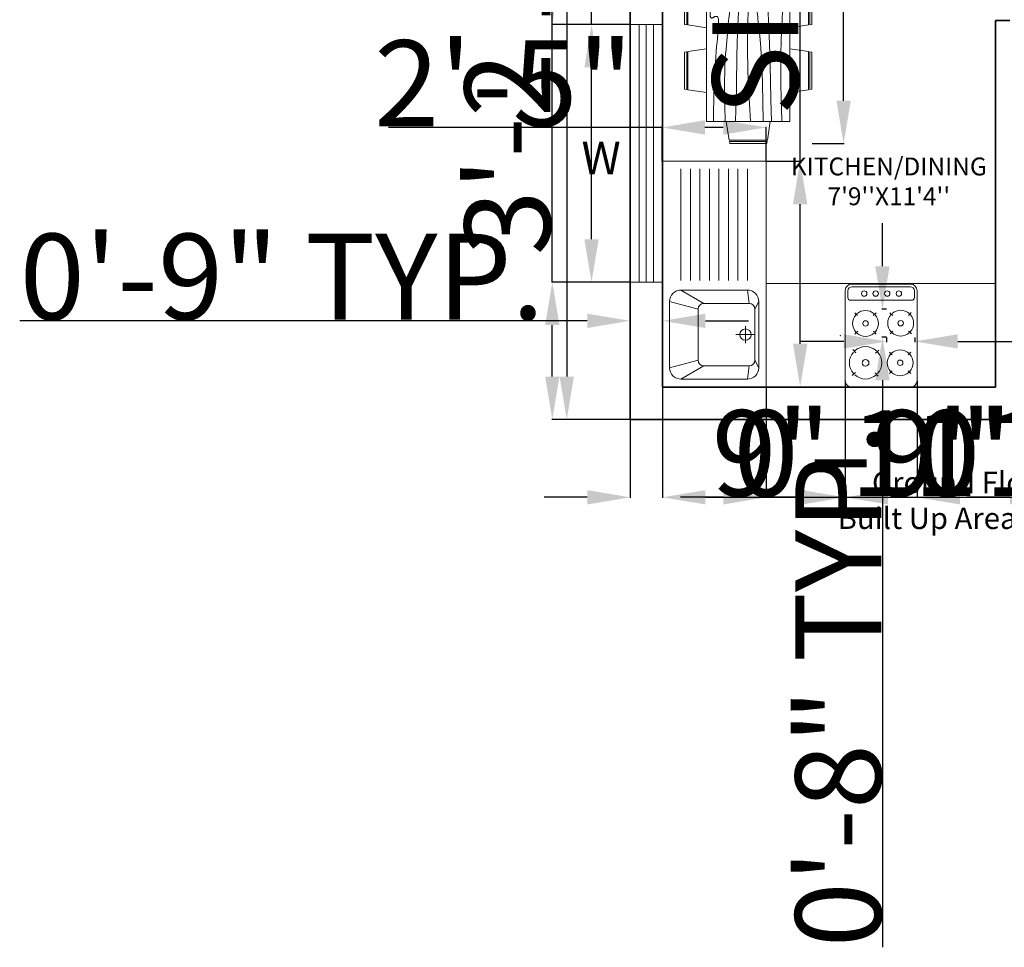
# Model space of a CAD drawing. Units: inches. Extents: x 2236 to 2927, y 1577 to 2452.
# Tile 1 of 9: x 2236 to 2511, y 1577 to 1836. Entities that reach past the tile are written whole.
import ezdxf

# ---------------------------------------------------------------- set-up
doc = ezdxf.new("R2010")
doc.units = ezdxf.units.IN
for name, color, linetype, lineweight in [('A-ANNO-DIMS', 2, 'Continuous', 18), ('A-ANNO-TEXT', 7, 'Continuous', 18), ('A-AREA-IDEN', 7, 'Continuous', 18), ('A-EQPM', 9, 'Continuous', 18), ('A-FLOR-CASE', 40, 'Continuous', 18), ('A-FLOR-FIXT', 9, 'Continuous', 18), ('A-FURN', 8, 'Continuous', 18), ('Wall', 7, 'Continuous', 35), ('Windows', 162, 'Continuous', 18)]:
    doc.layers.add(name, color=color, linetype=linetype, lineweight=lineweight)
doc.styles.get("Standard").update_dxf_attribs({"font": 'arial.ttf'})
doc.dimstyles.get("Standard").update_dxf_attribs({"dimtxt": 24, "dimasz": 12, "dimexe": 0.18, "dimexo": 0.0625, "dimgap": 0.09, "dimtad": 1, "dimdec": 1, "dimzin": 0, "dimdsep": 46, "dimlunit": 4, "dimtxsty": 'Standard', "dimcen": 0.09, "dimadec": 0, "dimazin": 0, "dimtfac": 1, "dimtdec": 1, "dimtofl": 0, "dimtmove": 0, "dimatfit": 3, "dimfxl": 1, "dimtolj": 1, "dimtzin": 0, "dimarcsym": 0})

# ---------------------------------------------------------------- blocks, each defined once
blk = doc.blocks.new('KK')
for p, q in [((0, 0.55), (0, 0)), ((1.19, 0.55), (0, 0.55)), ((1.19, 0), (1.19, 0.55)), ((0.1, 0.51), (0.14, 0.36)), ((0.45, 0.51), (0.1, 0.51)), ((0.41, 0.36), (0.45, 0.51)), ((0.11, 0.33), (0.04, 0.45)), ((0.04, 0.45), (0.04, 0.1)), ((0.44, 0.33), (0.51, 0.45)), ((0.51, 0.1), (0.51, 0.45)), ((0.56, 0.45), (1.15, 0.45)), ((0.56, 0.4), (1.15, 0.4)), ((0.11, 0.09), (0.11, 0.33)), ((0.14, 0.36), (0.41, 0.36)), ((0.44, 0.33), (0.44, 0.09)), ((0.56, 0.35), (1.15, 0.35)), ((0.56, 0.3), (1.15, 0.3)), ((0.56, 0.25), (1.15, 0.25)), ((0.275, 0.06), (0.275, 0.16)), ((0.56, 0.2), (1.15, 0.2)), ((0.23, 0.11), (0.32, 0.11)), ((0.56, 0.15), (1.15, 0.15)), ((0.04, 0.1), (0.11, 0.09)), ((0.14, 0.06), (0.1, 0.04)), ((0.41, 0.06), (0.14, 0.06)), ((0.41, 0.06), (0.45, 0.04)), ((0.44, 0.09), (0.51, 0.1)), ((0.56, 0.1), (1.15, 0.1)), ((0, 0), (1.19, 0)), ((0.1, 0.04), (0.45, 0.04))]:
    blk.add_line(p, q)
blk.add_circle((0.275, 0.11), 0.03)
for centre, radius, start, end in [((0.1, 0.45), 0.06, 90, 180), ((0.45, 0.45), 0.06, 0, 90), ((0.14, 0.33), 0.03, 90, 180), ((0.41, 0.33), 0.03, 0, 90), ((0.1, 0.1), 0.06, 180, 270), ((0.14, 0.09), 0.03, 180, 270), ((0.41, 0.09), 0.03, 270, 0), ((0.45, 0.1), 0.06, 270, 0)]:
    blk.add_arc(centre, radius, start, end)
blk = doc.blocks.new('Dining Set - 36 x 72 in.')
for p, q in [((-22.2343, 26.00059), (-23.4847, 17.99762)), ((-22.2304, 26), (-5.7608, 26)), ((-22, 27.5), (-22.1562, 26.50042)), ((-5.8416, 26.5), (-22.1534, 26.5)), ((-22, 27.5), (-6, 27.5)), ((-5.8437, 26.49966), (-6, 27.5)), ((-4.5152, 17.99762), (-5.7655, 25.99926)), ((5.7657, 26.00059), (4.5153, 17.99762)), ((5.7696, 26), (22.2392, 26)), ((6, 27.5), (5.8438, 26.50042)), ((22.1584, 26.5), (5.8466, 26.5)), ((6, 27.5), (22, 27.5)), ((22.1563, 26.49966), (22, 27.5)), ((23.4848, 17.99762), (22.2345, 25.99926)), ((36, 18), (-36, 18)), ((-36, 18), (-36, -18)), ((36, -18), (36, 18)), ((-44.0006, 8.23428), (-35.9976, 9.48474)), ((44.0006, 8.23428), (35.9976, 9.48474)), ((-45.5, 8), (-44.5004, 8.15617)), ((-45.5, 8), (-45.5, -8)), ((-44.5, -8.15843), (-44.5, 8.15338)), ((-44, 8.23041), (-44, -8.23915)), ((44, 8.23041), (44, -8.23915)), ((44.5, -8.15843), (44.5, 8.15338)), ((45.5, 8), (44.5005, 8.15617)), ((45.5, 8), (45.5, -8)), ((-44.4997, -8.15631), (-45.5, -8)), ((-35.9976, -9.48476), (-43.9993, -8.2345)), ((35.9976, -9.48476), (43.9993, -8.2345)), ((44.4997, -8.15631), (45.5, -8)), ((-36, -18), (36, -18)), ((-22.2343, -26.0006), (-23.4847, -17.99762)), ((-4.5152, -17.99762), (-5.7655, -25.99928)), ((5.7657, -26.0006), (4.5153, -17.99762)), ((23.4848, -17.99762), (22.2345, -25.99928)), ((-22.2304, -26), (-5.7608, -26)), ((-22, -27.5), (-22.1562, -26.50044)), ((-5.8416, -26.5), (-22.1534, -26.5)), ((-22, -27.5), (-6, -27.5)), ((-5.8437, -26.49967), (-6, -27.5)), ((5.7696, -26), (22.2392, -26)), ((6, -27.5), (5.8438, -26.50044)), ((22.1584, -26.5), (5.8466, -26.5)), ((6, -27.5), (22, -27.5)), ((22.1563, -26.49967), (22, -27.5))]:
    blk.add_line(p, q)
for points in [[(-36, 15), (-31.1772, 14.97754), (-26.8079, 14.91406), (-22.8538, 14.81543), (-19.276, 14.6875), (-16.0362, 14.53613), (-13.0957, 14.36718), (-10.4159, 14.18652), (-7.9583, 14), (-5.6904, 13.81315), (-3.6035, 13.63021), (-1.6954, 13.45508), (0.0365, 13.29166), (1.5945, 13.14388), (2.9811, 13.01562), (4.1988, 12.9108), (5.25, 12.83333), (6.1393, 12.78613), (6.8802, 12.76823), (7.4883, 12.77767), (7.9792, 12.8125), (8.3685, 12.87077), (8.6719, 12.95052), (8.9049, 13.0498), (9.0833, 13.16666), (9.2205, 13.29899), (9.3216, 13.44401), (9.3895, 13.59879), (9.4271, 13.76041), (9.4373, 13.92594), (9.4232, 14.09245), (9.3875, 14.257), (9.3333, 14.41666), (9.2638, 14.56917), (9.1836, 14.71484), (9.0975, 14.85465), (9.0104, 14.98958), (8.9272, 15.1206), (8.8529, 15.2487), (8.7922, 15.37483), (8.75, 15.5), (8.7305, 15.62467), (8.7344, 15.74739), (8.7617, 15.86621), (8.8125, 15.97916), (8.8867, 16.08431), (8.9844, 16.17968), (9.1055, 16.26334), (9.25, 16.33333), (9.4189, 16.38802), (9.6172, 16.42708), (9.8506, 16.45052), (10.125, 16.45833), (10.4463, 16.45052), (10.8203, 16.42708), (11.2529, 16.38802), (11.75, 16.33333), (12.3184, 16.26318), (12.9694, 16.17838), (13.7151, 16.07991), (14.5677, 15.96875), (15.5395, 15.84586), (16.6426, 15.71224), (17.8893, 15.56884), (19.2917, 15.41666), (20.859, 15.25667), (22.5879, 15.08984), (24.4721, 14.91715), (26.5052, 14.73958), (28.6809, 14.5581), (30.9929, 14.3737), (33.4347, 14.18733), (36, 14)], [(-36, 10), (-28.9766, 10.14274), (-23.1725, 10.20442), (-18.4241, 10.19775), (-14.5677, 10.13541), (-11.4399, 10.03011), (-8.877, 9.89453), (-6.7154, 9.74137), (-4.7917, 9.58333), (-2.9698, 9.43082), (-1.2246, 9.28515), (0.4415, 9.14534), (2.026, 9.01041), (3.5266, 8.87939), (4.9408, 8.7513), (6.266, 8.62516), (7.5, 8.5), (8.6411, 8.37549), (9.6914, 8.2539), (10.6538, 8.13818), (11.5312, 8.03125), (12.3267, 7.93603), (13.043, 7.85547), (13.6831, 7.79248), (14.25, 7.75), (14.7471, 7.7303), (15.1797, 7.73307), (15.5537, 7.75732), (15.875, 7.80208), (16.1494, 7.86637), (16.3828, 7.94922), (16.5811, 8.04964), (16.75, 8.16666), (16.8944, 8.29915), (17.0143, 8.44531), (17.1089, 8.60319), (17.1771, 8.77083), (17.218, 8.94629), (17.2305, 9.1276), (17.2137, 9.31282), (17.1667, 9.5), (17.0895, 9.6875), (16.987, 9.875), (16.8649, 10.0625), (16.7292, 10.25), (16.5856, 10.4375), (16.4401, 10.625), (16.2985, 10.8125), (16.1667, 11), (16.05, 11.18733), (15.9518, 11.3737), (15.8752, 11.5581), (15.8229, 11.73958), (15.798, 11.91715), (15.8034, 12.08984), (15.842, 12.25667), (15.9167, 12.41666), (16.0295, 12.56836), (16.1784, 12.70833), (16.3605, 12.83268), (16.5729, 12.9375), (16.8127, 13.01888), (17.0768, 13.07291), (17.3625, 13.0957), (17.6667, 13.08333), (17.9894, 13.03312), (18.3418, 12.94726), (18.7382, 12.82918), (19.1927, 12.68229), (19.7195, 12.51001), (20.3327, 12.31575), (21.0465, 12.10294), (21.875, 11.875), (22.8357, 11.63354), (23.959, 11.37304), (25.2786, 11.08618), (26.8282, 10.76562), (28.6414, 10.40405), (30.752, 9.99414), (33.1936, 9.52856), (36, 9)], [(-36, 5.5), (-30.7157, 5.3348), (-26.069, 5.20963), (-21.9946, 5.11767), (-18.4271, 5.05208), (-15.3009, 5.00602), (-12.5508, 4.97265), (-10.1112, 4.94515), (-7.9167, 4.91666), (-5.909, 4.88167), (-4.0586, 4.83984), (-2.3429, 4.79215), (-0.7396, 4.73958), (0.7739, 4.6831), (2.22, 4.6237), (3.6213, 4.56233), (5, 4.5), (6.373, 4.43782), (7.7344, 4.3776), (9.0723, 4.32129), (10.375, 4.27083), (11.6309, 4.22819), (12.8281, 4.19531), (13.9551, 4.17415), (15, 4.16666), (15.954, 4.17448), (16.819, 4.19791), (17.6001, 4.23698), (18.3021, 4.29166), (18.9299, 4.36198), (19.4883, 4.44791), (19.9823, 4.54948), (20.4167, 4.66666), (20.7969, 4.79899), (21.1302, 4.94401), (21.4245, 5.09879), (21.6875, 5.26041), (21.9271, 5.42594), (22.1511, 5.59245), (22.3672, 5.757), (22.5834, 5.91666), (22.8065, 6.06868), (23.0404, 6.21093), (23.2879, 6.34147), (23.5521, 6.45833), (23.8358, 6.55957), (24.142, 6.64323), (24.4735, 6.70735), (24.8334, 6.75), (25.2235, 6.76969), (25.642, 6.76692), (26.0858, 6.74267), (26.5521, 6.69791), (27.0379, 6.63362), (27.5404, 6.55078), (28.0565, 6.45036), (28.5834, 6.33333), (29.1242, 6.19987), (29.7071, 6.04687), (30.3661, 5.87044), (31.1354, 5.66666), (32.0493, 5.43164), (33.142, 5.16146), (34.4475, 4.85221), (36, 4.5)], [(-36, -1), (-30.7915, -0.6591), (-26.0195, -0.38216), (-21.6519, -0.16284), (-17.6563, 0.00521), (-14.0005, 0.12833), (-10.6523, 0.21289), (-7.5796, 0.26522), (-4.75, 0.29166), (-2.134, 0.29793), (0.2878, 0.28711), (2.5317, 0.26163), (4.6146, 0.22396), (6.5529, 0.17651), (8.3633, 0.12174), (10.0623, 0.06209), (11.6667, 0), (13.1899, -0.06201), (14.6341, -0.1211), (15.9982, -0.17432), (17.2813, -0.21875), (18.4823, -0.25147), (19.6003, -0.26953), (20.6343, -0.27002), (21.5834, -0.25), (22.4481, -0.20768), (23.2357, -0.14584), (23.9549, -0.06836), (24.6146, 0.02083), (25.2235, 0.11784), (25.7904, 0.21875), (26.3241, 0.31966), (26.8334, 0.41666), (27.3265, 0.50618), (27.8099, 0.58593), (28.2894, 0.65397), (28.7709, 0.70833), (29.2601, 0.74707), (29.763, 0.76823), (30.2855, 0.76985), (30.8334, 0.75), (31.4088, 0.70784), (31.9994, 0.64713), (32.589, 0.57275), (33.1615, 0.48958), (33.7008, 0.4025), (34.1908, 0.3164), (34.6153, 0.23616), (34.9584, 0.16666), (35.2099, 0.11165), (35.3848, 0.07031), (35.504, 0.04069), (35.5886, 0.02083), (35.6594, 0.00879), (35.7377, 0.0026), (35.8442, 0.00032), (36, 0)], [(-36, -6.5), (-27.1843, -6.31267), (-20.084, -6.1263), (-14.469, -5.9419), (-10.1094, -5.76042), (-6.7752, -5.58285), (-4.2363, -5.41016), (-2.2629, -5.24333), (-0.625, -5.08334), (0.8708, -4.93099), (2.2715, -4.78646), (3.5872, -4.64974), (4.8281, -4.52084), (6.0046, -4.39974), (7.127, -4.28646), (8.2053, -4.18099), (9.25, -4.08334), (10.2705, -3.99382), (11.2734, -3.91407), (12.2647, -3.84603), (13.25, -3.79167), (14.2354, -3.75293), (15.2266, -3.73177), (16.2295, -3.73015), (17.25, -3.75), (18.2912, -3.79248), (19.3451, -3.85547), (20.4009, -3.93604), (21.4479, -4.03125), (22.4754, -4.13819), (23.4727, -4.25391), (24.4289, -4.37549), (25.3334, -4.5), (26.1785, -4.62492), (26.9694, -4.74935), (27.7145, -4.87281), (28.4219, -4.99479), (29.1, -5.11483), (29.7572, -5.23242), (30.4016, -5.34709), (31.0417, -5.45834), (31.6837, -5.56437), (32.3262, -5.65821), (32.9658, -5.73153), (33.599, -5.77604), (34.2224, -5.78345), (34.8327, -5.74545), (35.4264, -5.65373), (36, -5.5)], [(-36, -10), (-26.4022, -9.81299), (-18.4675, -9.62891), (-11.9839, -9.45069), (-6.7396, -9.28125), (-2.5226, -9.12354), (0.8789, -8.98047), (3.6769, -8.85498), (6.0833, -8.75), (8.2767, -8.66765), (10.3021, -8.60677), (12.1712, -8.56543), (13.8958, -8.54167), (15.4876, -8.53353), (16.9583, -8.53907), (18.3197, -8.55632), (19.5834, -8.58334), (20.7616, -8.61841), (21.8685, -8.66081), (22.9188, -8.71004), (23.9271, -8.76563), (24.9081, -8.82707), (25.8763, -8.89388), (26.8465, -8.96558), (27.8334, -9.04167), (28.8474, -9.12118), (29.8828, -9.20117), (30.93, -9.27824), (31.9792, -9.34896), (33.0205, -9.40991), (34.0443, -9.45768), (35.0407, -9.48885), (36, -9.5)], [(-36, -14.5), (-30.0881, -14.33513), (-25.0332, -14.21224), (-20.7312, -14.12647), (-17.0781, -14.07292), (-13.97, -14.04671), (-11.3027, -14.04297), (-8.9724, -14.05681), (-6.875, -14.08334), (-4.9224, -14.11833), (-3.0905, -14.16016), (-1.3709, -14.20785), (0.2448, -14.26042), (1.7647, -14.3169), (3.1973, -14.3763), (4.5507, -14.43767), (5.8333, -14.5), (7.0554, -14.5621), (8.235, -14.62175), (9.3922, -14.67652), (10.5469, -14.72396), (11.7192, -14.76164), (12.929, -14.78711), (14.1965, -14.79794), (15.5417, -14.79167), (16.9933, -14.76424), (18.6152, -14.70508), (20.4804, -14.60197), (22.6615, -14.44271), (25.2312, -14.21509), (28.2624, -13.9069), (31.8277, -13.50594), (36, -13)]]:
    blk.add_lwpolyline(points)
blk = doc.blocks.new('*D10')
at = {"layer": 'A-ANNO-DIMS', "color": 0, "lineweight": -2, "transparency": 16777216}
for p, q in [((2406.79, 2084.08), (2388.95, 2084.08)), ((2389.13, 2072.08), (2389.13, 1736.08)), ((2406.79, 1724.08), (2388.95, 1724.08))]:
    blk.add_line(p, q, dxfattribs=at)
at = {"layer": 'A-ANNO-DIMS', "color": 0, "transparency": 16777216}
for points in [[(2387.13, 2072.08), (2391.13, 2072.08), (2389.13, 2084.08)], [(2387.13, 1736.08), (2391.13, 1736.08), (2389.13, 1724.08)]]:
    blk.add_solid(points, dxfattribs=at)
at = {"layer": 'Defpoints', "color": 0, "transparency": 16777216}
for p in [(2406.85, 2084.08), (2389.13, 1724.08), (2406.85, 1724.08)]:
    blk.add_point(p, dxfattribs=at)
at = {"layer": 'A-ANNO-DIMS', "color": 0, "transparency": 16777216, "insert": (2376.78, 1904.08), "char_height": 24, "attachment_point": 5, "rotation": 90}
blk.add_mtext("\\A1;30'", dxfattribs=at)
blk = doc.blocks.new('WIN-72IN')
for p, q in [((0, 6.5), (72, 6.5)), ((0, 4.5), (72, 4.5)), ((0, 2.5), (72, 2.5))]:
    blk.add_line(p, q)
blk.add_lwpolyline([(0, 9), (72, 9), (72, 0), (0, 0)], close=True)
blk = doc.blocks.new('COOKTOP-BURNER')
for p, q in [((0.6, 6.56), (1.41, 5.8)), ((6.56, 6.61), (5.8, 5.81)), ((0.66, 0.6), (1.41, 1.41)), ((6.61, 0.66), (5.81, 1.41))]:
    blk.add_line(p, q)
blk.add_circle((3.61, 3.61), 0.759)
for start, end in [(138.017, 221.983), (48.017, 131.983), (318.017, 41.983), (228.017, 311.983)]:
    blk.add_arc((3.61, 3.61), 3.61, start, end)
blk = doc.blocks.new('*D18')
at = {"layer": 'A-ANNO-DIMS', "color": 0, "lineweight": -2, "transparency": 16777216}
for p, q in [((2396.05, 1834.44), (2396.05, 2191.28)), ((2406.79, 1834.44), (2395.87, 1834.44)), ((2396.05, 1774.44), (2396.05, 1822.44)), ((2406.79, 1762.44), (2395.87, 1762.44))]:
    blk.add_line(p, q, dxfattribs=at)
at = {"layer": 'A-ANNO-DIMS', "color": 0, "transparency": 16777216}
for points in [[(2394.05, 1822.44), (2398.05, 1822.44), (2396.05, 1834.44)], [(2394.05, 1774.44), (2398.05, 1774.44), (2396.05, 1762.44)]]:
    blk.add_solid(points, dxfattribs=at)
at = {"layer": 'Defpoints', "color": 0, "transparency": 16777216}
for p in [(2396.05, 1834.44), (2406.85, 1834.44), (2406.85, 1762.44)]:
    blk.add_point(p, dxfattribs=at)
at = {"layer": 'A-ANNO-DIMS', "color": 0, "transparency": 16777216, "insert": (2383.54, 2018.86), "char_height": 24, "attachment_point": 5, "rotation": 90}
blk.add_mtext('\\A1;WINDOW W 6\'-0" TYP.', dxfattribs=at)
blk = doc.blocks.new('*D19')
at = {"layer": 'A-ANNO-DIMS', "color": 0, "lineweight": -2, "transparency": 16777216}
for p, q in [((2406.85, 1762.38), (2406.85, 1751.46)), ((2415.85, 1762.38), (2415.85, 1751.46)), ((2394.85, 1751.64), (2236.38, 1751.64)), ((2427.85, 1751.64), (2439.85, 1751.64))]:
    blk.add_line(p, q, dxfattribs=at)
at = {"layer": 'A-ANNO-DIMS', "color": 0, "transparency": 16777216}
for points in [[(2394.85, 1753.64), (2394.85, 1749.64), (2406.85, 1751.64)], [(2427.85, 1753.64), (2427.85, 1749.64), (2415.85, 1751.64)]]:
    blk.add_solid(points, dxfattribs=at)
at = {"layer": 'Defpoints', "color": 0, "transparency": 16777216}
for p in [(2406.85, 1762.44), (2415.85, 1762.44), (2406.85, 1751.64)]:
    blk.add_point(p, dxfattribs=at)
at = {"layer": 'A-ANNO-DIMS', "color": 0, "transparency": 16777216, "insert": (2309.61, 1763.98), "char_height": 24, "attachment_point": 5}
blk.add_mtext('\\A1;0\'-9" TYP.', dxfattribs=at)
blk = doc.blocks.new('*D24')
at = {"layer": 'A-ANNO-DIMS', "color": 0, "lineweight": -2, "transparency": 16777216}
for p, q in [((2466.46, 1745.89), (2454.46, 1745.89)), ((2478.46, 1747), (2478.46, 1745.71)), ((2486.29, 1747), (2486.29, 1745.71)), ((2498.29, 1745.89), (2806.59, 1745.89))]:
    blk.add_line(p, q, dxfattribs=at)
at = {"layer": 'A-ANNO-DIMS', "color": 0, "transparency": 16777216}
for points in [[(2466.46, 1747.89), (2466.46, 1743.89), (2478.46, 1745.89)], [(2498.29, 1747.89), (2498.29, 1743.89), (2486.29, 1745.89)]]:
    blk.add_solid(points, dxfattribs=at)
at = {"layer": 'Defpoints', "color": 0, "transparency": 16777216}
for p in [(2478.46, 1747.06), (2486.29, 1747.06), (2486.29, 1745.89)]:
    blk.add_point(p, dxfattribs=at)
at = {"layer": 'A-ANNO-DIMS', "color": 0, "transparency": 16777216, "insert": (2658.44, 1758.23), "char_height": 24, "attachment_point": 5}
blk.add_mtext('\\A1;BURNER 0\'-8" TYP.', dxfattribs=at)
blk = doc.blocks.new('*D25')
at = {"layer": 'A-ANNO-DIMS', "color": 0, "lineweight": -2, "transparency": 16777216}
for p, q in [((2477.28, 1766.89), (2477.28, 1778.89)), ((2478.39, 1754.89), (2477.1, 1754.89)), ((2478.39, 1747.06), (2477.1, 1747.06)), ((2477.28, 1735.06), (2477.28, 1576.59))]:
    blk.add_line(p, q, dxfattribs=at)
at = {"layer": 'A-ANNO-DIMS', "color": 0, "transparency": 16777216}
for points in [[(2475.28, 1766.89), (2479.28, 1766.89), (2477.28, 1754.89)], [(2475.28, 1735.06), (2479.28, 1735.06), (2477.28, 1747.06)]]:
    blk.add_solid(points, dxfattribs=at)
at = {"layer": 'Defpoints', "color": 0, "transparency": 16777216}
for p in [(2478.46, 1754.89), (2477.28, 1747.06), (2478.46, 1747.06)]:
    blk.add_point(p, dxfattribs=at)
at = {"layer": 'A-ANNO-DIMS', "color": 0, "transparency": 16777216, "insert": (2464.94, 1649.83), "char_height": 24, "attachment_point": 5, "rotation": 90}
blk.add_mtext('\\A1;0\'-8" TYP.', dxfattribs=at)
blk = doc.blocks.new('*D36')
at = {"layer": 'A-ANNO-DIMS', "color": 0, "lineweight": -2, "transparency": 16777216}
for p, q in [((2454.3, 1796.23), (2454.3, 2047.2)), ((2444.91, 1796.23), (2454.48, 1796.23)), ((2454.3, 1745.23), (2454.3, 1784.23)), ((2444.91, 1733.23), (2454.48, 1733.23))]:
    blk.add_line(p, q, dxfattribs=at)
at = {"layer": 'A-ANNO-DIMS', "color": 0, "transparency": 16777216}
for points in [[(2452.3, 1784.23), (2456.3, 1784.23), (2454.3, 1796.23)], [(2452.3, 1745.23), (2456.3, 1745.23), (2454.3, 1733.23)]]:
    blk.add_solid(points, dxfattribs=at)
at = {"layer": 'Defpoints', "color": 0, "transparency": 16777216}
for p in [(2444.85, 1796.23), (2454.3, 1796.23), (2444.85, 1733.23)]:
    blk.add_point(p, dxfattribs=at)
at = {"layer": 'A-ANNO-DIMS', "color": 0, "transparency": 16777216, "insert": (2441.79, 1927.72), "char_height": 24, "attachment_point": 5, "rotation": 90}
blk.add_mtext('\\A1;SINK UNIT 5\'-3"', dxfattribs=at)
blk = doc.blocks.new('*D37')
at = {"layer": 'A-ANNO-DIMS', "color": 0, "lineweight": -2, "transparency": 16777216}
for p, q in [((2415.73, 1805.68), (2339.34, 1805.68)), ((2415.73, 1796.29), (2415.73, 1805.86)), ((2432.85, 1805.68), (2427.73, 1805.68)), ((2444.85, 1796.29), (2444.85, 1805.86))]:
    blk.add_line(p, q, dxfattribs=at)
at = {"layer": 'A-ANNO-DIMS', "color": 0, "transparency": 16777216}
for points in [[(2427.73, 1807.68), (2427.73, 1803.68), (2415.73, 1805.68)], [(2432.85, 1807.68), (2432.85, 1803.68), (2444.85, 1805.68)]]:
    blk.add_solid(points, dxfattribs=at)
at = {"layer": 'Defpoints', "color": 0, "transparency": 16777216}
for p in [(2415.73, 1805.68), (2415.73, 1796.23), (2444.85, 1796.23)]:
    blk.add_point(p, dxfattribs=at)
at = {"layer": 'A-ANNO-DIMS', "color": 0, "transparency": 16777216, "insert": (2371.53, 1818.03), "char_height": 24, "attachment_point": 5}
blk.add_mtext('\\A1;2\'-5"', dxfattribs=at)
blk = doc.blocks.new('*D38')
at = {"layer": 'A-ANNO-DIMS', "color": 0, "lineweight": -2, "transparency": 16777216}
for p, q in [((2466.44, 1860.06), (2466.44, 2154.67)), ((2457.67, 1860.06), (2466.62, 1860.06)), ((2466.44, 1813.15), (2466.44, 1848.06)), ((2457.67, 1801.15), (2466.62, 1801.15))]:
    blk.add_line(p, q, dxfattribs=at)
at = {"layer": 'A-ANNO-DIMS', "color": 0, "transparency": 16777216}
for points in [[(2464.44, 1848.06), (2468.44, 1848.06), (2466.44, 1860.06)], [(2464.44, 1813.15), (2468.44, 1813.15), (2466.44, 1801.15)]]:
    blk.add_solid(points, dxfattribs=at)
at = {"layer": 'Defpoints', "color": 0, "transparency": 16777216}
for p in [(2457.61, 1860.06), (2466.44, 1860.06), (2457.61, 1801.15)]:
    blk.add_point(p, dxfattribs=at)
at = {"layer": 'A-ANNO-DIMS', "color": 0, "transparency": 16777216, "insert": (2453.94, 2013.36), "char_height": 24, "attachment_point": 5, "rotation": 90}
blk.add_mtext('\\A1;DINING SET 4\'-11"', dxfattribs=at)
blk = doc.blocks.new('*D43')
at = {"layer": 'A-ANNO-DIMS', "color": 0, "lineweight": -2, "transparency": 16777216}
for p, q in [((2385.1, 1893.71), (2385.1, 2045.22)), ((2406.79, 1893.71), (2384.92, 1893.71)), ((2385.1, 1846.44), (2385.1, 1881.71)), ((2406.79, 1834.44), (2384.92, 1834.44))]:
    blk.add_line(p, q, dxfattribs=at)
at = {"layer": 'A-ANNO-DIMS', "color": 0, "transparency": 16777216}
for points in [[(2383.1, 1881.71), (2387.1, 1881.71), (2385.1, 1893.71)], [(2383.1, 1846.44), (2387.1, 1846.44), (2385.1, 1834.44)]]:
    blk.add_solid(points, dxfattribs=at)
at = {"layer": 'Defpoints', "color": 0, "transparency": 16777216}
for p in [(2385.1, 1893.71), (2406.85, 1893.71), (2406.85, 1834.44)]:
    blk.add_point(p, dxfattribs=at)
at = {"layer": 'A-ANNO-DIMS', "color": 0, "transparency": 16777216, "insert": (2372.6, 1975.46), "char_height": 24, "attachment_point": 5, "rotation": 90}
blk.add_mtext('\\A1;4\'-11 1/2"', dxfattribs=at)
blk = doc.blocks.new('*D44')
at = {"layer": 'A-ANNO-DIMS', "color": 0, "lineweight": -2, "transparency": 16777216}
for p, q in [((2385.1, 1762.44), (2385.1, 1894.33)), ((2406.79, 1762.44), (2384.92, 1762.44)), ((2385.1, 1736.08), (2385.1, 1750.44)), ((2406.79, 1724.08), (2384.92, 1724.08))]:
    blk.add_line(p, q, dxfattribs=at)
at = {"layer": 'A-ANNO-DIMS', "color": 0, "transparency": 16777216}
for points in [[(2383.1, 1750.44), (2387.1, 1750.44), (2385.1, 1762.44)], [(2383.1, 1736.08), (2387.1, 1736.08), (2385.1, 1724.08)]]:
    blk.add_solid(points, dxfattribs=at)
at = {"layer": 'Defpoints', "color": 0, "transparency": 16777216}
for p in [(2385.1, 1762.44), (2406.85, 1762.44), (2406.85, 1724.08)]:
    blk.add_point(p, dxfattribs=at)
at = {"layer": 'A-ANNO-DIMS', "color": 0, "transparency": 16777216, "insert": (2372.59, 1834.38), "char_height": 24, "attachment_point": 5, "rotation": 90}
blk.add_mtext('\\A1;3\'-2 1/2"', dxfattribs=at)
blk = doc.blocks.new('*D46')
at = {"layer": 'A-ANNO-DIMS', "color": 0, "lineweight": -2, "transparency": 16777216}
for p, q in [((2415.85, 1873.01), (2415.85, 1702.15)), ((2533.86, 1873.01), (2533.86, 1702.15)), ((2427.85, 1702.33), (2521.86, 1702.33))]:
    blk.add_line(p, q, dxfattribs=at)
at = {"layer": 'A-ANNO-DIMS', "color": 0, "transparency": 16777216}
for points in [[(2427.85, 1704.33), (2427.85, 1700.33), (2415.85, 1702.33)], [(2521.86, 1704.33), (2521.86, 1700.33), (2533.86, 1702.33)]]:
    blk.add_solid(points, dxfattribs=at)
at = {"layer": 'Defpoints', "color": 0, "transparency": 16777216}
for p in [(2415.85, 1873.08), (2533.86, 1873.08), (2533.86, 1702.33)]:
    blk.add_point(p, dxfattribs=at)
at = {"layer": 'A-ANNO-DIMS', "color": 0, "transparency": 16777216, "insert": (2474.85, 1714.67), "char_height": 24, "attachment_point": 5}
blk.add_mtext('\\A1;9\'-10"', dxfattribs=at)
blk = doc.blocks.new('*D48')
at = {"layer": 'A-ANNO-DIMS', "color": 0, "lineweight": -2, "transparency": 16777216}
for p, q in [((2524.86, 1915.51), (2524.86, 1702.15)), ((2533.86, 1915.51), (2533.86, 1702.15)), ((2512.86, 1702.33), (2500.86, 1702.33)), ((2545.86, 1702.33), (2621.84, 1702.33))]:
    blk.add_line(p, q, dxfattribs=at)
at = {"layer": 'A-ANNO-DIMS', "color": 0, "transparency": 16777216}
for points in [[(2512.86, 1704.33), (2512.86, 1700.33), (2524.86, 1702.33)], [(2545.86, 1704.33), (2545.86, 1700.33), (2533.86, 1702.33)]]:
    blk.add_solid(points, dxfattribs=at)
at = {"layer": 'Defpoints', "color": 0, "transparency": 16777216}
for p in [(2524.86, 1915.58), (2533.86, 1915.58), (2533.86, 1702.33)]:
    blk.add_point(p, dxfattribs=at)
at = {"layer": 'A-ANNO-DIMS', "color": 0, "transparency": 16777216, "insert": (2589.85, 1714.67), "char_height": 24, "attachment_point": 5}
blk.add_mtext('\\A1;0\'-9"', dxfattribs=at)
blk = doc.blocks.new('*D49')
at = {"layer": 'A-ANNO-DIMS', "color": 0, "lineweight": -2, "transparency": 16777216}
for p, q in [((2415.85, 1733.01), (2415.85, 1702.15)), ((2406.85, 1724.01), (2406.85, 1702.15)), ((2394.85, 1702.33), (2382.85, 1702.33)), ((2427.85, 1702.33), (2503.83, 1702.33))]:
    blk.add_line(p, q, dxfattribs=at)
at = {"layer": 'A-ANNO-DIMS', "color": 0, "transparency": 16777216}
for points in [[(2394.85, 1704.33), (2394.85, 1700.33), (2406.85, 1702.33)], [(2427.85, 1704.33), (2427.85, 1700.33), (2415.85, 1702.33)]]:
    blk.add_solid(points, dxfattribs=at)
at = {"layer": 'Defpoints', "color": 0, "transparency": 16777216}
for p in [(2415.85, 1733.08), (2406.85, 1724.08), (2415.85, 1702.33)]:
    blk.add_point(p, dxfattribs=at)
at = {"layer": 'A-ANNO-DIMS', "color": 0, "transparency": 16777216, "insert": (2471.84, 1714.67), "char_height": 24, "attachment_point": 5}
blk.add_mtext('\\A1;0\'-9"', dxfattribs=at)
blk = doc.blocks.new('*D58')
at = {"layer": 'A-ANNO-DIMS', "color": 0, "lineweight": -2, "transparency": 16777216}
for p, q in [((2466.86, 1734.91), (2466.86, 1702.15)), ((2486.98, 1734.91), (2486.98, 1702.15)), ((2454.86, 1702.33), (2442.86, 1702.33)), ((2498.98, 1702.33), (2572.7, 1702.33))]:
    blk.add_line(p, q, dxfattribs=at)
at = {"layer": 'A-ANNO-DIMS', "color": 0, "transparency": 16777216}
for points in [[(2454.86, 1704.33), (2454.86, 1700.33), (2466.86, 1702.33)], [(2498.98, 1704.33), (2498.98, 1700.33), (2486.98, 1702.33)]]:
    blk.add_solid(points, dxfattribs=at)
at = {"layer": 'Defpoints', "color": 0, "transparency": 16777216}
for p in [(2466.86, 1734.97), (2486.98, 1734.97), (2486.98, 1702.33)]:
    blk.add_point(p, dxfattribs=at)
at = {"layer": 'A-ANNO-DIMS', "color": 0, "transparency": 16777216, "insert": (2541.84, 1714.67), "char_height": 24, "attachment_point": 5}
blk.add_mtext('\\A1;1\'-8"', dxfattribs=at)
blk = doc.blocks.new('*D59')
at = {"layer": 'A-ANNO-DIMS', "color": 0, "lineweight": -2, "transparency": 16777216}
for p, q in [((2466.86, 1734.91), (2466.86, 1702.15)), ((2444.85, 1733.17), (2444.85, 1702.15)), ((2432.85, 1702.33), (2420.85, 1702.33)), ((2478.86, 1702.33), (2571.23, 1702.33))]:
    blk.add_line(p, q, dxfattribs=at)
at = {"layer": 'A-ANNO-DIMS', "color": 0, "transparency": 16777216}
for points in [[(2432.85, 1704.33), (2432.85, 1700.33), (2444.85, 1702.33)], [(2478.86, 1704.33), (2478.86, 1700.33), (2466.86, 1702.33)]]:
    blk.add_solid(points, dxfattribs=at)
at = {"layer": 'Defpoints', "color": 0, "transparency": 16777216}
for p in [(2466.86, 1734.97), (2444.85, 1733.23), (2466.86, 1702.33)]:
    blk.add_point(p, dxfattribs=at)
at = {"layer": 'A-ANNO-DIMS', "color": 0, "transparency": 16777216, "insert": (2531.04, 1714.67), "char_height": 24, "attachment_point": 5}
blk.add_mtext('\\A1;1\'-10"', dxfattribs=at)

msp = doc.modelspace()

# ---------------------------------------------------------------- linework, layer by layer
at = {"layer": 'A-EQPM'}
for p, q in [((2466.86, 1760.03), (2466.86, 1734.97)), ((2467.62, 1760.03), (2467.62, 1758.14)), ((2485.08, 1761.93), (2468.76, 1761.93)), ((2485.08, 1761.17), (2468.76, 1761.17)), ((2486.22, 1758.14), (2486.22, 1760.03)), ((2486.98, 1734.97), (2486.98, 1760.03)), ((2468.38, 1757.38), (2485.46, 1757.38)), ((2469.56, 1753.89), (2470.36, 1753.09)), ((2475.52, 1753.92), (2474.73, 1753.12)), ((2469.59, 1747.92), (2470.38, 1748.73)), ((2475.55, 1747.96), (2474.75, 1748.75)), ((2468.99, 1743.61), (2469.83, 1742.71)), ((2476.25, 1743.48), (2475.36, 1742.64)), ((2468.86, 1736.35), (2469.75, 1737.18)), ((2476.12, 1736.21), (2475.28, 1737.11)), ((2468.76, 1733.08), (2485.08, 1733.08))]:
    msp.add_line(p, q, dxfattribs=at)
for centre, radius in [((2472.18, 1759.27), 0.759), ((2475.4, 1759.27), 0.759), ((2478.63, 1759.27), 0.759), ((2481.86, 1759.27), 0.759), ((2472.56, 1750.92), 0.759), ((2472.56, 1739.91), 0.952)]:
    msp.add_circle(centre, radius, dxfattribs=at)
for centre, radius, start, end in [((2468.76, 1760.03), 1.9, 90, 180), ((2468.76, 1760.03), 1.14, 90, 180), ((2485.08, 1760.03), 1.9, 0, 90), ((2485.08, 1760.03), 1.14, 0, 90), ((2468.38, 1758.14), 0.759, 180, 270), ((2485.46, 1758.14), 0.759, 270, 0), ((2472.56, 1750.92), 3.61, 48.017, 131.983), ((2472.56, 1750.92), 3.61, 138.017, 221.983), ((2472.56, 1750.92), 3.61, 318.017, 41.983), ((2472.56, 1750.92), 3.61, 228.017, 311.983), ((2472.56, 1739.91), 4.52, 48.017, 131.983), ((2472.56, 1739.91), 4.52, 138.017, 221.983), ((2472.56, 1739.91), 4.52, 318.017, 41.983), ((2468.76, 1734.97), 1.9, 180, 270), ((2472.56, 1739.91), 4.52, 228.017, 311.983), ((2485.08, 1734.97), 1.9, 270, 0)]:
    msp.add_arc(centre, radius, start, end, dxfattribs=at)
msp.add_point((2465.53, 1747.5), dxfattribs=at)
at = {"layer": 'A-FLOR-CASE'}
for p, q in [((2444.85, 1796.23), (2444.85, 1762.08)), ((2444.85, 1762.08), (2508.85, 1762.08))]:
    msp.add_line(p, q, dxfattribs=at)
at = {"layer": 'Wall'}
for p, q in [((2406.85, 2084.08), (2406.85, 1724.08)), ((2415.85, 1869.08), (2415.85, 1733.08)), ((2508.85, 1835.53), (2512.85, 1835.53)), ((2508.85, 1835.53), (2508.85, 1733.08)), ((2415.85, 1733.08), (2508.85, 1733.08)), ((2406.85, 1724.08), (2622.85, 1724.08))]:
    msp.add_line(p, q, dxfattribs=at)

# ---------------------------------------------------------------- block references
at = {"layer": 'A-EQPM', "rotation": 269.9999999998117}
msp.add_blockref('COOKTOP-BURNER', (2478.76, 1754.58), dxfattribs=at)
at = {"layer": 'A-EQPM'}
msp.add_blockref('COOKTOP-BURNER', (2478.63, 1736.3), dxfattribs=at)
at = {"layer": 'A-FLOR-FIXT', "xscale": 52.94470845768636, "yscale": 52.94470845768636, "zscale": 52.94470845768636, "rotation": 90}
msp.add_blockref('KK', (2444.85, 1733.23), dxfattribs=at)
at = {"layer": 'A-FURN', "xscale": 0.6472934063691596, "yscale": 0.6472934063691596, "zscale": 0.6472934063691596, "rotation": 90}
msp.add_blockref('Dining Set - 36 x 72 in.', (2439.81, 1830.6), dxfattribs=at)
at = {"layer": 'Windows', "rotation": 90.00000000000259}
msp.add_blockref('WIN-72IN', (2415.85, 1762.44), dxfattribs=at)

# ---------------------------------------------------------------- texts
at = {"layer": 'A-ANNO-TEXT'}
msp.add_text('W', height=9.12, dxfattribs=at).set_placement((2393.27, 1792.55))
at = {"layer": 'A-ANNO-TEXT', "insert": (2428.34, 1709.48), "char_height": 6, "attachment_point": 1}
msp.add_mtext_dynamic_manual_height_columns('\\pxqc;Ground Floor Plan\\PBuilt Up Area : 540sq.ft.', width=161.5717, gutter_width=45.58, heights=[0], dxfattribs=at)
at = {"layer": 'A-AREA-IDEN', "insert": (2460.35, 1797.28), "char_height": 5, "attachment_point": 1}
msp.add_mtext_dynamic_manual_height_columns("\\pxqc;KITCHEN/DINING\\P7'9''X11'4''", width=37.4353, gutter_width=12.5, heights=[0], dxfattribs=at)

# ---------------------------------------------------------------- dimensions: what is measured, and where the dimension line sits
at = {"layer": 'A-ANNO-DIMS'}
for base, p1, p2, angle, text, picture, middle in [((2396.05, 1834.44), (2406.85, 1762.44), (2406.85, 1834.44), 90, 'WINDOW W <> TYP.', '*D18', (2383.54, 2018.86)), ((2466.44, 1860.06), (2457.61, 1801.15), (2457.61, 1860.06), 90, 'DINING SET <>', '*D38', (2453.94, 2013.36)), ((2454.3, 1796.23), (2444.85, 1733.23), (2444.85, 1796.23), 90, 'SINK UNIT <>', '*D36', (2441.79, 1927.72)), ((2406.85, 1751.64), (2415.85, 1762.44), (2406.85, 1762.44), 180, '<> TYP.', '*D19', (2309.61, 1763.98)), ((2477.28, 1747.06), (2478.46, 1754.89), (2478.46, 1747.06), 270, '<> TYP.', '*D25', (2464.94, 1649.83))]:
    dim = msp.add_linear_dim(base=base, p1=p1, p2=p2, angle=angle, text=text, dimstyle='Standard', override={"dimdec": 1, "dimlfac": 1, "dimrnd": 0, "dimzin": 1, "dimdsep": 46, "dimlunit": 4, "dimfrac": 2}, dxfattribs=at)
    dim.commit()
    dim.dimension.update_dxf_attribs({"geometry": picture, "text_midpoint": middle})
for base, p1, p2, angle, override, picture, middle in [((2389.13, 1724.08), (2406.85, 2084.08), (2406.85, 1724.08), 90, {"dimclrd": 0, "dimclre": 0, "dimclrt": 0}, '*D10', (2376.78, 1904.08)), ((2385.1, 1893.71), (2406.85, 1834.44), (2406.85, 1893.71), 90, {"dimdec": 1, "dimlfac": 1, "dimrnd": 0, "dimzin": 1, "dimdsep": 46, "dimlunit": 4, "dimfrac": 2}, '*D43', (2372.6, 1975.46)), ((2385.1, 1762.44), (2406.85, 1724.08), (2406.85, 1762.44), 90, {"dimdec": 1, "dimlfac": 1, "dimrnd": 0, "dimzin": 1, "dimdsep": 46, "dimlunit": 4, "dimfrac": 2}, '*D44', (2372.59, 1834.38)), ((2415.73, 1805.68), (2444.85, 1796.23), (2415.73, 1796.23), 180, {"dimdec": 1, "dimlfac": 1, "dimrnd": 0, "dimzin": 1, "dimdsep": 46, "dimlunit": 4, "dimfrac": 2}, '*D37', (2371.53, 1818.03))]:
    dim = msp.add_linear_dim(base=base, p1=p1, p2=p2, angle=angle, dimstyle='Standard', override=override, dxfattribs=at)
    dim.commit()
    dim.dimension.update_dxf_attribs({"geometry": picture, "text_midpoint": middle})
for base, p1, p2, picture, middle in [((2533.86, 1702.33), (2524.86, 1915.58), (2533.86, 1915.58), '*D48', (2589.85, 1714.67)), ((2533.86, 1702.33), (2415.85, 1873.08), (2533.86, 1873.08), '*D46', (2474.85, 1714.67)), ((2466.86, 1702.33), (2444.85, 1733.23), (2466.86, 1734.97), '*D59', (2531.04, 1714.67)), ((2486.98, 1702.33), (2466.86, 1734.97), (2486.98, 1734.97), '*D58', (2541.84, 1714.67)), ((2415.85, 1702.33), (2406.85, 1724.08), (2415.85, 1733.08), '*D49', (2471.84, 1714.67))]:
    dim = msp.add_linear_dim(base=base, p1=p1, p2=p2, dimstyle='Standard', override={"dimdec": 1, "dimlfac": 1, "dimrnd": 0, "dimzin": 1, "dimdsep": 46, "dimlunit": 4, "dimfrac": 2}, dxfattribs=at)
    dim.commit()
    dim.dimension.update_dxf_attribs({"geometry": picture, "text_midpoint": middle})
dim = msp.add_linear_dim(base=(2486.29, 1745.89), p1=(2478.46, 1747.06), p2=(2486.29, 1747.06), text='BURNER <> TYP.', dimstyle='Standard', override={"dimdec": 1, "dimlfac": 1, "dimrnd": 0, "dimzin": 1, "dimdsep": 46, "dimlunit": 4, "dimfrac": 2}, dxfattribs=at)
dim.commit()
dim.dimension.update_dxf_attribs({"geometry": '*D24', "text_midpoint": (2658.44, 1758.23)})

doc.saveas('drawing.dxf')
